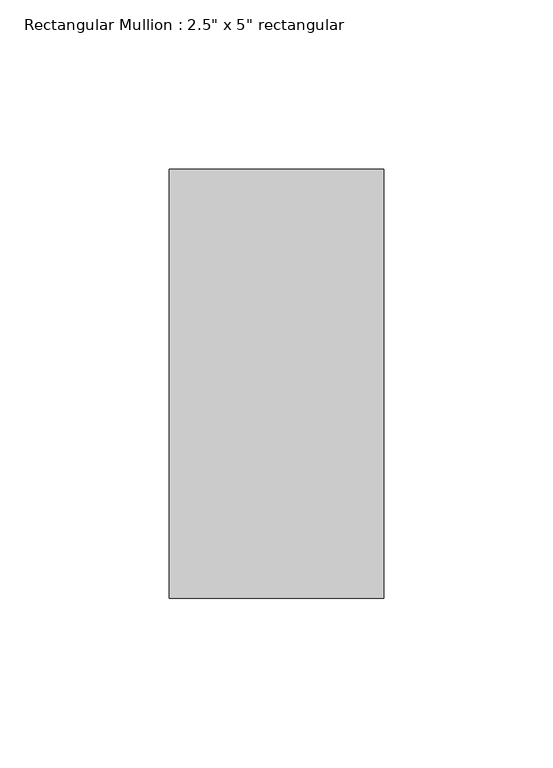
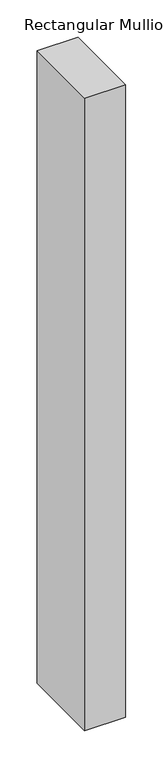
"""IFC4 building model written with IfcOpenShell, lengths in millimetres: member geometry."""

from ifc_helpers import new_model, si_unit, frame, origin, place, context, project, spatial, polyline, outline, extrude, source, transform, mapped, element, save


def member_4a65f4ca(model_context):
    return source(origin(), model_context, "Body", "SweptSolid", [
        extrude(outline(polyline([(0.0, 63.5), (0.0, -63.5), (-63.5, -63.5), (-63.5, 63.5), (0.0, 63.5)])), frame((0.0, 0.0, -1032.9333333), z_axis=(0.0, 0.0, 1.0), x_axis=(1.0, 0.0, 0.0)), (0.0, 0.0, 1.0), 1032.9333333),
    ])


if __name__ == "__main__":
    model = new_model("IFC4")
    model_context = context("Model", 3, world=origin())
    ifc_project = project(units=[si_unit("LENGTHUNIT", "METRE", prefix="MILLI")], contexts=[model_context])
    site = spatial("IfcSite", under=ifc_project)
    building = spatial("IfcBuilding", under=site)
    placement = place(None, origin())
    member_shape = member_4a65f4ca(model_context)
    element("IfcMember", 1, ObjectType="Rectangular Mullion : 2.5\" x 5\" rectangular", at=placement, inside=building, context=model_context, shape_type="MappedRepresentation", body=[
        mapped(member_shape, transform((0.0, 0.0, 0.0), x_axis=(1.0, 0.0, 0.0), y_axis=(0.0, 1.0, 0.0), z_axis=(0.0, 0.0, 1.0))),
    ])
    save(model, "model.ifc")

# Revit data of these elements
# Type "Rectangular Mullion : 2.5\" x 5\" rectangular"
#   built-in parameter 1007304 = 0.416667 (stored number, unit not read)
#   built-in parameter 1007301 = 0.104167 (stored number, unit not read)
#   built-in parameter 1007300 = 0.104167 (stored number, unit not read)
# Element 1 (IfcMember, "Rectangular Mullion : 2.5\" x 5\" rectangular")
#   Materials on its faces: "Aluminum"
# Materials
#   "Aluminum": class "Metal", colour RGB 247 247 247, transparency 0, Description = "Aluminum 6061", Cost = 0
